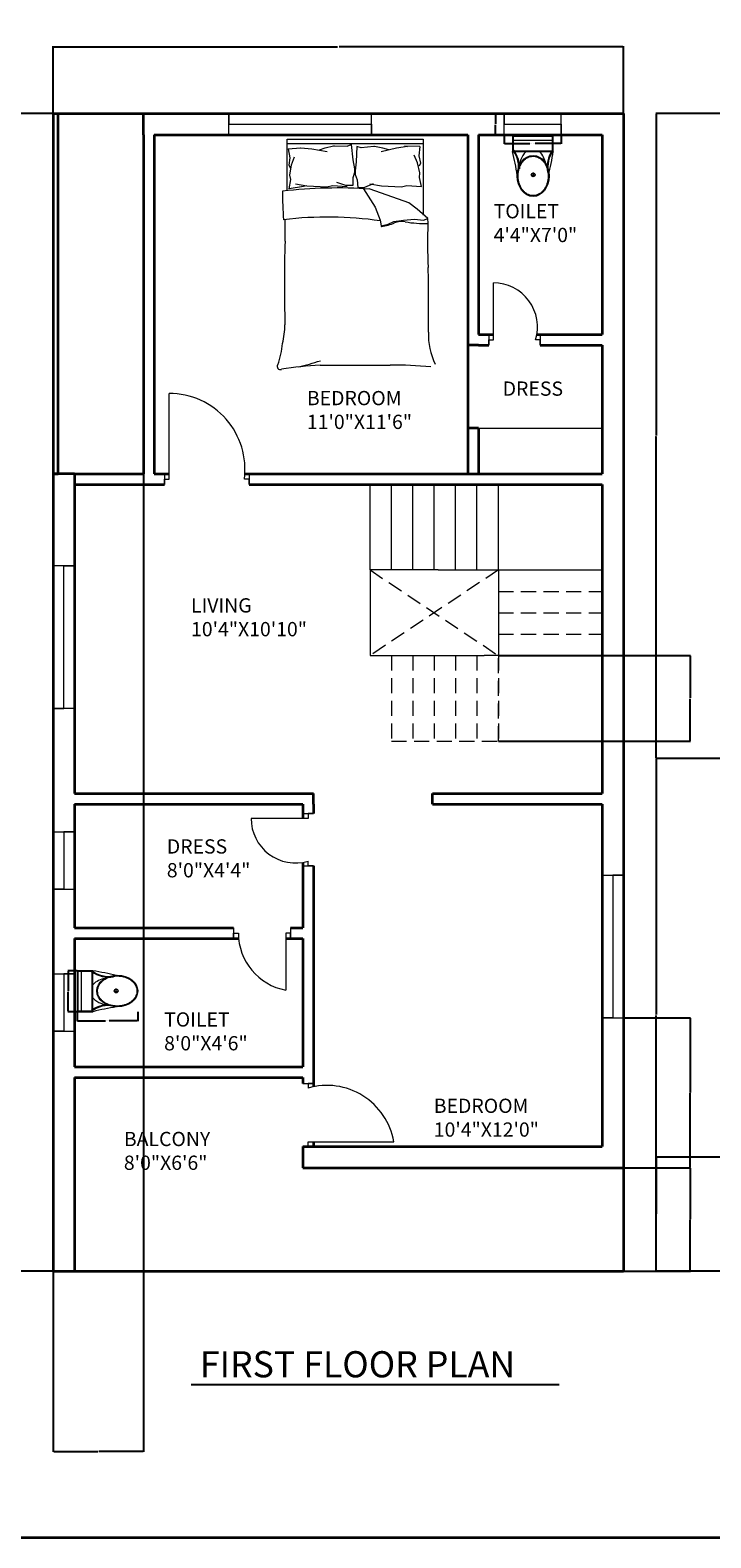
# Model space of a CAD drawing. Units: inches. Extents: x 1911 to 3278, y 2022 to 3108.
# Tile 9 of 13: x 2298 to 2585, y 2022 to 2656. Entities that reach past the tile are written whole.
import ezdxf

# ---------------------------------------------------------------- set-up
doc = ezdxf.new("R2010")
doc.units = ezdxf.units.IN
doc.linetypes.add('DASHED2', pattern=[9.525, 6.35, -3.175])
for name, color, linetype, lineweight in [('A-ANNO-DIMS', 2, 'Continuous', 18), ('A-ANNO-TITL', 7, 'Continuous', 25), ('A-ANNO-TTLB', 7, 'Continuous', 35), ('A-AREA-IDEN', 7, 'Continuous', 18), ('A-DOOR', 4, 'Continuous', 18), ('A-FLOR-CASE', 9, 'Continuous', 18), ('A-FLOR-FIXT', 9, 'Continuous', 18), ('A-FLOR-STRS', 7, 'Continuous', 18), ('A-FLOR-STRS-OVHD', 253, 'DASHED2', 13), ('A-FURN', 8, 'Continuous', 13), ('A-GLAZ', 4, 'Continuous', 18), ('A-WALL', 7, 'Continuous', 35)]:
    doc.layers.add(name, color=color, linetype=linetype, lineweight=lineweight)
doc.styles.get("Standard").update_dxf_attribs({"font": 'arial.ttf'})
doc.dimstyles.get("Standard").update_dxf_attribs({"dimtxt": 0.18, "dimasz": 0.18, "dimexe": 0.18, "dimexo": 0.0625, "dimgap": 0.09, "dimtad": 0, "dimtih": 1, "dimtoh": 1, "dimdec": 4, "dimzin": 0, "dimdsep": 46, "dimtxsty": 'Standard', "dimcen": 0.09, "dimadec": 0, "dimazin": 0, "dimtfac": 1, "dimtdec": 4, "dimtofl": 0, "dimtmove": 0, "dimatfit": 3, "dimfxl": 1, "dimtolj": 1, "dimtzin": 0, "dimarcsym": 0})

# ---------------------------------------------------------------- blocks, each defined once
blk = doc.blocks.new('A$C31115884')
for p, q in [((283, 498), (223, 498)), ((258, 466), (258, 523)), ((0, 200), (0, 0)), ((520, 200), (0, 200)), ((520, 0), (520, 200)), ((510, 54), (0, 54)), ((10, 190), (10, 10)), ((510, 190), (10, 190)), ((10, 10), (510, 10)), ((510, 10), (510, 190)), ((0, 0), (520, 0))]:
    blk.add_line(p, q)
blk.add_circle((256, 496), 23.6)
for centre, radius, start, end in [((2778, -205), 2807, 165.4549, 171.7133), ((-295, 403), 365, 324.2091, 9.3499), ((-295, 403), 375, 324.2091, 9.3499), ((139, 406), 293, 315.8436, 2.6563), ((806, 403), 375, 179.2036, 215.7909), ((806, 403), 365, 170.6501, 215.7909), ((3237, 905), 2807, 188.2867, 194.5451), ((384, 406), 293, 190.2774, 224.1564)]:
    blk.add_arc(centre, radius, start, end)
blk.add_ellipse((256, 510), major_axis=(0, -261), ratio=0.772727)
blk.add_open_spline([(256, 259), (263, 259), (270, 260), (288, 262), (299, 265), (320, 273), (330, 278), (350, 291), (360, 299), (378, 316), (386, 326), (402, 347), (409, 358), (421, 383), (427, 395), (436, 422), (440, 436), (445, 465), (447, 480), (448, 509), (448, 524), (445, 553), (443, 568), (436, 596), (432, 610), (422, 636), (416, 649), (402, 672), (395, 683), (379, 703), (370, 712), (351, 728), (341, 735), (321, 746), (310, 751), (289, 757), (278, 759), (256, 761), (245, 761), (223, 757), (212, 754), (191, 746), (181, 741), (161, 728), (151, 720), (133, 703), (125, 693), (110, 672), (103, 660), (90, 636), (85, 623), (76, 596), (72, 582), (67, 553), (66, 538), (64, 509), (65, 494), (68, 465), (70, 450), (77, 422), (81, 408), (91, 382), (97, 370), (111, 346), (118, 335), (135, 316), (144, 307), (162, 291), (172, 284), (193, 273), (203, 269), (225, 262), (236, 260), (250, 259), (253, 259), (256, 259)], degree=3, knots=[0, 0, 0, 0, 0.110105, 0.110105, 0.285049, 0.285049, 0.459994, 0.459994, 0.634938, 0.634938, 0.809882, 0.809882, 0.984827, 0.984827, 1.159771, 1.159771, 1.334715, 1.334715, 1.50966, 1.50966, 1.684604, 1.684604, 1.859549, 1.859549, 2.034493, 2.034493, 2.209437, 2.209437, 2.384382, 2.384382, 2.559326, 2.559326, 2.73427, 2.73427, 2.909215, 2.909215, 3.084159, 3.084159, 3.259103, 3.259103, 3.434048, 3.434048, 3.608992, 3.608992, 3.783936, 3.783936, 3.958881, 3.958881, 4.133825, 4.133825, 4.30877, 4.30877, 4.483714, 4.483714, 4.658658, 4.658658, 4.833603, 4.833603, 5.008547, 5.008547, 5.183491, 5.183491, 5.358436, 5.358436, 5.53338, 5.53338, 5.708324, 5.708324, 5.883269, 5.883269, 6.058213, 6.058213, 6.233158, 6.233158, 6.283185, 6.283185, 6.283185, 6.283185])
blk = doc.blocks.new('WIN-60')
for p, q in [((0, 60), (9, 60)), ((9, 60), (4.5, 60)), ((4.5, 60), (4.5, 0)), ((4.5, 0), (0, 0)), ((0, 0), (9, 0))]:
    blk.add_line(p, q)
blk = doc.blocks.new('WIN-24')
for p, q in [((0, 24), (9, 24)), ((9, 24), (4.5, 24)), ((4.5, 24), (4.5, 0)), ((4.5, 0), (0, 0)), ((0, 0), (9, 0))]:
    blk.add_line(p, q)
blk = doc.blocks.new('DOOR-BED-FF')
for p, q in [((2, 2.25), (2, 38.25)), ((0, 4.5), (0, 0)), ((0, 0), (0, 2.25)), ((0, 2.25), (2, 2.25)), ((35.66, 2.25), (33.66, 2.25)), ((35.66, 4.5), (35.66, 0)), ((35.66, 0), (35.66, 2.25))]:
    blk.add_line(p, q)
blk.add_arc((2, 6.33), 31.92, 352.65052, 90)
blk = doc.blocks.new('DOOR-BATH-FF')
for p, q in [((2, 2.25), (2, 26.25)), ((0, 4.5), (0, 0)), ((0, 0), (0, 2.25)), ((0, 2.25), (2, 2.25)), ((21.7, 2.25), (19.7, 2.25)), ((21.7, 4.5), (21.7, 0)), ((21.7, 0), (21.7, 2.25))]:
    blk.add_line(p, q)
blk.add_arc((2, 7.72), 18.53, 342.82983, 90)
blk = doc.blocks.new('DOOR-BALCONY')
for p, q in [((0, 26.53), (4.5, 26.53)), ((4.5, 26.53), (2.25, 26.53)), ((2.25, 26.53), (2.25, 24.53)), ((2.32, 0), (2.32, 2)), ((2.32, 2), (38.32, 2))]:
    blk.add_line(p, q)
blk.add_arc((10.23, -2.83), 28.5, 9.76334, 106.26632)
blk = doc.blocks.new('DOOR-DRESS-FF')
for p, q in [((24, 20), (0, 20)), ((21.75, 22), (26.25, 22)), ((26.25, 22), (24, 22)), ((24, 22), (24, 20)), ((21.75, 0), (26.25, 0)), ((24, 0), (24, 2)), ((26.25, 0), (24, 0))]:
    blk.add_line(p, q)
blk.add_arc((18.75, 20), 18.75, 180, 286.25091)
blk = doc.blocks.new('DOOR-ENSUITE-FF')
for p, q in [((0, 26.25), (0, 21.75)), ((23.93, 26.25), (23.93, 21.75)), ((0, 21.75), (0, 24)), ((0, 24), (0, 24)), ((0, 24), (2, 24)), ((23.93, 24), (21.93, 24)), ((21.93, 24), (21.93, 0)), ((23.93, 21.75), (23.93, 24))]:
    blk.add_line(p, q)
blk.add_arc((26.42, 24), 24.42, 180, 259.41225)
blk = doc.blocks.new('BED-DOUBLE')
for p, q in [((4.17, 75.16), (4.17, 96.87)), ((4.17, 96.87), (61.46, 96.87)), ((61.46, 96.87), (61.46, 64.97)), ((4.17, 95.03), (61.46, 95.03)), ((4.67, 92.87), (9.81, 93.27)), ((4.67, 92.9), (5.36, 89.08)), ((5.36, 89.08), (4.84, 85.96)), ((6.06, 86.14), (7.27, 89.43)), ((9.81, 93.27), (9.93, 93.24)), ((9.93, 93.24), (14.52, 92.9)), ((14.52, 92.9), (21.1, 91.68)), ((17.81, 92.38), (20.24, 93.24)), ((20.24, 93.24), (23.7, 94.11)), ((23.7, 94.11), (24.09, 94.11)), ((24.09, 94.11), (29.42, 93.94)), ((29.42, 93.94), (31.15, 94.63)), ((31.15, 94.63), (31.84, 88.22)), ((33.54, 93.88), (33.25, 87.44)), ((35.31, 93.3), (33.54, 93.88)), ((40.62, 93.81), (35.31, 93.3)), ((41.01, 93.83), (40.62, 93.81)), ((44.52, 93.18), (41.01, 93.83)), ((50.25, 93.19), (43.75, 91.57)), ((47, 92.47), (44.52, 93.18)), ((54.8, 93.82), (50.25, 93.19)), ((60.08, 93.81), (53.6, 93.92)), ((53.6, 93.92), (54.8, 93.82)), ((59.12, 86.97), (57.7, 90.18)), ((60.08, 93.81), (59.62, 89.96)), ((59.62, 89.96), (60.34, 86.88)), ((4.84, 85.96), (5.54, 84.75)), ((5.36, 81.8), (6.06, 86.14)), ((31.84, 88.22), (32.54, 84.4)), ((32.54, 82.84), (31.84, 80.59)), ((32.54, 84.4), (32.54, 82.84)), ((33.25, 87.44), (32.79, 83.59)), ((32.79, 83.59), (32.89, 82.03)), ((60.08, 82.69), (59.12, 86.97)), ((60.34, 86.88), (59.72, 85.62)), ((59.85, 80.77), (60.08, 82.69)), ((5.02, 76.08), (5.71, 79.9)), ((11.13, 76.95), (5.02, 76.08)), ((5.71, 79.9), (5.36, 81.8)), ((7.65, 78.14), (12.48, 77.34)), ((12.48, 77.34), (11.13, 76.95)), ((12.48, 77.34), (20.89, 76.82)), ((20.89, 76.82), (23.24, 77.49)), ((23.24, 77.49), (29.39, 77)), ((28.9, 77.37), (25.13, 78.68)), ((31.84, 77.37), (28.9, 77.37)), ((31.84, 80.59), (31.84, 77.37)), ((32.89, 82.03), (33.72, 79.83)), ((33.72, 79.83), (33.93, 76.62)), ((33.93, 76.62), (36.87, 76.8)), ((36.87, 76.8), (40.55, 78.34)), ((39.04, 78.14), (43.87, 77.34)), ((43.87, 77.34), (52.28, 76.82)), ((52.28, 76.82), (54.63, 77.49)), ((54.63, 77.49), (60.78, 77)), ((60.78, 77), (59.85, 80.77)), ((36.28, 76.03), (41.3, 68.25)), ((48.73, 72.52), (38.73, 76.03)), ((55.41, 70.1), (48.73, 72.52)), ((58.94, 67.51), (55.41, 70.1)), ((41.3, 68.25), (43.34, 62.87)), ((63.38, 63.61), (58.94, 67.51)), ((61.54, 62.87), (63.38, 63.61)), ((63.48, 61.52), (63.38, 63.61, 4.64)), ((43.34, 62.87), (43.71, 60.45)), ((43.71, 60.45), (46.68, 61.2)), ((46.68, 61.2), (49.1, 62.31)), ((49.1, 62.31), (53.18, 62.87)), ((53.18, 62.87), (57.82, 63.24)), ((57.82, 63.24), (61.54, 62.87)), ((18.06, 1.87), (47.57, 1.87))]:
    blk.add_line(p, q)
for centre, radius, start, end in [((25.61, -121.38), 197.77, 86.08655, 96.78213), ((102.1, 72.78), 99.87, 178.72178, 185.60397), ((21.29, -90.53), 154.68, 81.78449, 96.90062), ((-200.58, 59.5), 203.94, 358.4762, 1.00819), ((43.92, 60.38), 0.221, 160.24637, 271.13765), ((37.35, 95.1), 35.55, 280.66171, 289.88058), ((52.44, 54.83), 7.46, 78.6608, 113.73842), ((61.53, 104.85), 43.38, 259.87628, 272.56571), ((218.51, 53.34), 155.25, 176.97912, 183.83645), ((581.23, 36.19), 578.22, 178.22771, 181.71854), ((-5405.34, 15.56), 5469.02, 0.00217, 0.28689), ((-32.25, 19.53), 35.53, 346.06484, 358.91125), ((91.3, 14.55), 27.65, 177.47136, 206.46809), ((-25.97, 12.62), 28.25, 337.97508, 356.652), ((1.3, 1.3), 1.31, 146.17358, 293.47814), ((25.69, -143.9), 145.97, 92.99578, 99.40907), ((-20.65, 125.3), 127.63, 283.38322, 287.70533), ((49.34, -157.62), 159.5, 84.4998, 90.63509)]:
    blk.add_arc(centre, radius, start, end)
blk = doc.blocks.new('STAIR-PLAN-FF')
for p, q in [((0, 36), (0, 72)), ((9, 36), (9, 72)), ((18, 36), (18, 72)), ((27, 36), (27, 72)), ((36, 36), (36, 72)), ((45, 36), (45, 72)), ((54, 36), (54, 72)), ((28.63, 36), (0, 36)), ((0, 36), (0, 0)), ((28.63, 36), (97.65, 36)), ((54, 36), (54, 0)), ((54, 36), (54, 27)), ((0, 0), (48, 0)), ((54, 0), (48, 0))]:
    blk.add_line(p, q)
blk = doc.blocks.new('STAIR-BEYOND-FF')
for p, q in [((54, 72), (0, 36)), ((0, 72), (54, 36)), ((54, 72), (54, 63)), ((54, 63), (97.65, 63)), ((54, 54), (97.65, 54)), ((54, 45), (97.65, 45)), ((9, 36), (9, 0)), ((18, 36), (18, 0)), ((27, 36), (27, 0)), ((36, 36), (36, 0)), ((45, 36), (45, 0)), ((54, 36), (97.65, 36)), ((54, 0), (54, 36)), ((54, 36), (54, 0)), ((9, 0), (54, 0))]:
    blk.add_line(p, q)
blk = doc.blocks.new('*D26')
at = {"layer": 'A-ANNO-DIMS', "color": 0, "lineweight": -2, "transparency": 16777216}
for p, q in [((2497.89, 2611.81), (2497.89, 2608.09)), ((2498.07, 2608.27), (2508.77, 2608.27)), ((2521.71, 2608.27), (2511.01, 2608.27)), ((2521.89, 2611.81), (2521.89, 2608.09))]:
    blk.add_line(p, q, dxfattribs=at)
at = {"layer": 'A-ANNO-DIMS', "color": 0, "transparency": 16777216}
for points in [[(2498.07, 2608.3), (2498.07, 2608.24), (2497.89, 2608.27)], [(2521.71, 2608.3), (2521.71, 2608.24), (2521.89, 2608.27)]]:
    blk.add_solid(points, dxfattribs=at)
at = {"layer": 'Defpoints', "color": 0, "transparency": 16777216}
for p in [(2497.89, 2611.87), (2497.89, 2608.27), (2521.89, 2611.87)]:
    blk.add_point(p, dxfattribs=at)
at = {"layer": 'A-ANNO-DIMS', "color": 0, "transparency": 16777216, "insert": (2509.89, 2608.27), "char_height": 0.18, "attachment_point": 5}
blk.add_mtext('\\A1;WINDOW 24 TYP.', dxfattribs=at)
blk = doc.blocks.new('*D27')
at = {"layer": 'A-ANNO-DIMS', "color": 0, "lineweight": -2, "transparency": 16777216}
for p, q in [((2497.83, 2620.87), (2494.11, 2620.87)), ((2494.29, 2620.69), (2494.29, 2616.56)), ((2494.29, 2612.05), (2494.29, 2616.19)), ((2497.83, 2611.87), (2494.11, 2611.87))]:
    blk.add_line(p, q, dxfattribs=at)
at = {"layer": 'A-ANNO-DIMS', "color": 0, "transparency": 16777216}
for points in [[(2494.26, 2620.69), (2494.32, 2620.69), (2494.29, 2620.87)], [(2494.26, 2612.05), (2494.32, 2612.05), (2494.29, 2611.87)]]:
    blk.add_solid(points, dxfattribs=at)
at = {"layer": 'Defpoints', "color": 0, "transparency": 16777216}
for p in [(2494.29, 2620.87), (2497.89, 2620.87), (2497.89, 2611.87)]:
    blk.add_point(p, dxfattribs=at)
at = {"layer": 'A-ANNO-DIMS', "color": 0, "transparency": 16777216, "insert": (2494.29, 2616.37), "char_height": 0.18, "attachment_point": 5}
blk.add_mtext('\\A1;9 TYP.', dxfattribs=at)
blk = doc.blocks.new('*D34')
at = {"layer": 'A-ANNO-DIMS', "color": 0, "lineweight": -2, "transparency": 16777216}
for p, q in [((2318.18, 2242.98), (2318.18, 2239.04)), ((2318.36, 2239.22), (2330.15, 2239.22)), ((2343.48, 2239.22), (2331.7, 2239.22)), ((2343.66, 2242.98), (2343.66, 2239.04))]:
    blk.add_line(p, q, dxfattribs=at)
at = {"layer": 'A-ANNO-DIMS', "color": 0, "transparency": 16777216}
for points in [[(2318.36, 2239.25), (2318.36, 2239.19), (2318.18, 2239.22)], [(2343.48, 2239.25), (2343.48, 2239.19), (2343.66, 2239.22)]]:
    blk.add_solid(points, dxfattribs=at)
at = {"layer": 'Defpoints', "color": 0, "transparency": 16777216}
for p in [(2318.18, 2243.04), (2343.66, 2243.04), (2343.66, 2239.22)]:
    blk.add_point(p, dxfattribs=at)
at = {"layer": 'A-ANNO-DIMS', "color": 0, "transparency": 16777216, "insert": (2330.92, 2239.22), "char_height": 0.18, "attachment_point": 5}
blk.add_mtext('\\A1;WC 25 TYP.', dxfattribs=at)
blk = doc.blocks.new('*D35')
at = {"layer": 'A-ANNO-DIMS', "color": 0, "lineweight": -2, "transparency": 16777216}
for p, q in [((2318.12, 2260.24), (2314.18, 2260.24)), ((2314.36, 2260.06), (2314.36, 2251.82)), ((2314.36, 2243.22), (2314.36, 2251.46)), ((2318.12, 2243.04), (2314.18, 2243.04))]:
    blk.add_line(p, q, dxfattribs=at)
at = {"layer": 'A-ANNO-DIMS', "color": 0, "transparency": 16777216}
for points in [[(2314.33, 2260.06), (2314.39, 2260.06), (2314.36, 2260.24)], [(2314.33, 2243.22), (2314.39, 2243.22), (2314.36, 2243.04)]]:
    blk.add_solid(points, dxfattribs=at)
at = {"layer": 'Defpoints', "color": 0, "transparency": 16777216}
for p in [(2318.18, 2260.24), (2314.36, 2243.04), (2318.18, 2243.04)]:
    blk.add_point(p, dxfattribs=at)
at = {"layer": 'A-ANNO-DIMS', "color": 0, "transparency": 16777216, "insert": (2314.36, 2251.64), "char_height": 0.18, "attachment_point": 5}
blk.add_mtext('\\A1;17 TYP.', dxfattribs=at)
blk = doc.blocks.new('*D75')
at = {"layer": 'A-ANNO-DIMS', "color": 0, "lineweight": -2, "transparency": 16777216}
for p, q in [((2308.12, 2620.94), (2308.12, 2649.15)), ((2308.3, 2648.97), (2427.83, 2648.97)), ((2547.94, 2648.97), (2428.41, 2648.97)), ((2548.12, 2620.94), (2548.12, 2649.15))]:
    blk.add_line(p, q, dxfattribs=at)
at = {"layer": 'A-ANNO-DIMS', "color": 0, "transparency": 16777216}
for points in [[(2308.3, 2649), (2308.3, 2648.94), (2308.12, 2648.97)], [(2547.94, 2649), (2547.94, 2648.94), (2548.12, 2648.97)]]:
    blk.add_solid(points, dxfattribs=at)
at = {"layer": 'Defpoints', "color": 0, "transparency": 16777216}
for p in [(2548.12, 2648.97), (2308.12, 2620.87), (2548.12, 2620.87)]:
    blk.add_point(p, dxfattribs=at)
at = {"layer": 'A-ANNO-DIMS', "color": 0, "transparency": 16777216, "insert": (2428.12, 2648.97), "char_height": 0.18, "attachment_point": 5}
blk.add_mtext('\\A1;240', dxfattribs=at)
blk = doc.blocks.new('*D76')
at = {"layer": 'A-ANNO-DIMS', "color": 0, "lineweight": -2, "transparency": 16777216}
for p, q in [((2308.06, 2620.87), (2279.84, 2620.87)), ((2280.02, 2620.69), (2280.02, 2377.56)), ((2280.02, 2134.05), (2280.02, 2377.19)), ((2308.06, 2133.87), (2279.84, 2133.87))]:
    blk.add_line(p, q, dxfattribs=at)
at = {"layer": 'A-ANNO-DIMS', "color": 0, "transparency": 16777216}
for points in [[(2279.99, 2620.69), (2280.05, 2620.69), (2280.02, 2620.87)], [(2279.99, 2134.05), (2280.05, 2134.05), (2280.02, 2133.87)]]:
    blk.add_solid(points, dxfattribs=at)
at = {"layer": 'Defpoints', "color": 0, "transparency": 16777216}
for p in [(2280.02, 2620.87), (2308.12, 2620.87), (2308.12, 2133.87)]:
    blk.add_point(p, dxfattribs=at)
at = {"layer": 'A-ANNO-DIMS', "color": 0, "transparency": 16777216, "insert": (2280.02, 2377.37), "char_height": 0.18, "attachment_point": 5}
blk.add_mtext('\\A1;487', dxfattribs=at)
blk = doc.blocks.new('*D77')
at = {"layer": 'A-ANNO-DIMS', "color": 0, "lineweight": -2, "transparency": 16777216}
for p, q in [((2308.12, 2620.81), (2308.12, 2057.89)), ((2346.12, 2620.81), (2346.12, 2057.89)), ((2308.3, 2058.07), (2326.9, 2058.07)), ((2345.94, 2058.07), (2327.34, 2058.07))]:
    blk.add_line(p, q, dxfattribs=at)
at = {"layer": 'A-ANNO-DIMS', "color": 0, "transparency": 16777216}
for points in [[(2308.3, 2058.1), (2308.3, 2058.04), (2308.12, 2058.07)], [(2345.94, 2058.1), (2345.94, 2058.04), (2346.12, 2058.07)]]:
    blk.add_solid(points, dxfattribs=at)
at = {"layer": 'Defpoints', "color": 0, "transparency": 16777216}
for p in [(2308.12, 2620.87), (2346.12, 2620.87), (2346.12, 2058.07)]:
    blk.add_point(p, dxfattribs=at)
at = {"layer": 'A-ANNO-DIMS', "color": 0, "transparency": 16777216, "insert": (2327.12, 2058.07), "char_height": 0.18, "attachment_point": 5}
blk.add_mtext('\\A1;38', dxfattribs=at)
blk = doc.blocks.new('*D78')
at = {"layer": 'A-ANNO-DIMS', "color": 0, "lineweight": -2, "transparency": 16777216}
for p, q in [((2548.18, 2177.37), (2576.4, 2177.37)), ((2576.22, 2177.19), (2576.22, 2155.81)), ((2576.22, 2134.05), (2576.22, 2155.44)), ((2548.18, 2133.87), (2576.4, 2133.87))]:
    blk.add_line(p, q, dxfattribs=at)
at = {"layer": 'A-ANNO-DIMS', "color": 0, "transparency": 16777216}
for points in [[(2576.19, 2177.19), (2576.25, 2177.19), (2576.22, 2177.37)], [(2576.19, 2134.05), (2576.25, 2134.05), (2576.22, 2133.87)]]:
    blk.add_solid(points, dxfattribs=at)
at = {"layer": 'Defpoints', "color": 0, "transparency": 16777216}
for p in [(2548.12, 2177.37), (2576.22, 2177.37), (2548.12, 2133.87)]:
    blk.add_point(p, dxfattribs=at)
at = {"layer": 'A-ANNO-DIMS', "color": 0, "transparency": 16777216, "insert": (2576.22, 2155.62), "char_height": 0.18, "attachment_point": 5}
blk.add_mtext('\\A1;43.5', dxfattribs=at)
blk = doc.blocks.new('*D79')
at = {"layer": 'A-ANNO-DIMS', "color": 0, "lineweight": -2, "transparency": 16777216}
for p, q in [((2548.18, 2240.47), (2576.4, 2240.47)), ((2576.22, 2240.29), (2576.22, 2209.1)), ((2576.22, 2177.55), (2576.22, 2208.74)), ((2548.18, 2177.37), (2576.4, 2177.37))]:
    blk.add_line(p, q, dxfattribs=at)
at = {"layer": 'A-ANNO-DIMS', "color": 0, "transparency": 16777216}
for points in [[(2576.19, 2240.29), (2576.25, 2240.29), (2576.22, 2240.47)], [(2576.19, 2177.55), (2576.25, 2177.55), (2576.22, 2177.37)]]:
    blk.add_solid(points, dxfattribs=at)
at = {"layer": 'Defpoints', "color": 0, "transparency": 16777216}
for p in [(2548.12, 2240.47), (2576.22, 2240.47), (2548.12, 2177.37)]:
    blk.add_point(p, dxfattribs=at)
at = {"layer": 'A-ANNO-DIMS', "color": 0, "transparency": 16777216, "insert": (2576.22, 2208.92), "char_height": 0.18, "attachment_point": 5}
blk.add_mtext('\\A1;63.09', dxfattribs=at)
blk = doc.blocks.new('*D80')
at = {"layer": 'A-ANNO-DIMS', "color": 0, "lineweight": -2, "transparency": 16777216}
for p, q in [((2495.53, 2392.87), (2576.4, 2392.87)), ((2576.22, 2392.69), (2576.22, 2375.06)), ((2576.22, 2357.05), (2576.22, 2374.69)), ((2495.53, 2356.87), (2576.4, 2356.87))]:
    blk.add_line(p, q, dxfattribs=at)
at = {"layer": 'A-ANNO-DIMS', "color": 0, "transparency": 16777216}
for points in [[(2576.19, 2392.69), (2576.25, 2392.69), (2576.22, 2392.87)], [(2576.19, 2357.05), (2576.25, 2357.05), (2576.22, 2356.87)]]:
    blk.add_solid(points, dxfattribs=at)
at = {"layer": 'Defpoints', "color": 0, "transparency": 16777216}
for p in [(2495.47, 2392.87), (2495.47, 2356.87), (2576.22, 2356.87)]:
    blk.add_point(p, dxfattribs=at)
at = {"layer": 'A-ANNO-DIMS', "color": 0, "transparency": 16777216, "insert": (2576.22, 2374.87), "char_height": 0.18, "attachment_point": 5}
blk.add_mtext('\\A1;36', dxfattribs=at)
blk = doc.blocks.new('*D83')
at = {"layer": 'A-ANNO-DIMS', "color": 0, "lineweight": -2, "transparency": 16777216}
for p, q in [((2633.29, 2620.87), (2561.76, 2620.87)), ((2561.94, 2620.69), (2561.94, 2485.38)), ((2561.94, 2349.71), (2561.94, 2485.02)), ((2593.28, 2349.53), (2561.76, 2349.53))]:
    blk.add_line(p, q, dxfattribs=at)
at = {"layer": 'A-ANNO-DIMS', "color": 0, "transparency": 16777216}
for points in [[(2561.91, 2620.69), (2561.97, 2620.69), (2561.94, 2620.87)], [(2561.91, 2349.71), (2561.97, 2349.71), (2561.94, 2349.53)]]:
    blk.add_solid(points, dxfattribs=at)
at = {"layer": 'Defpoints', "color": 0, "transparency": 16777216}
for p in [(2561.94, 2620.87), (2633.35, 2620.87), (2593.34, 2349.53)]:
    blk.add_point(p, dxfattribs=at)
at = {"layer": 'A-ANNO-DIMS', "color": 0, "transparency": 16777216, "insert": (2561.94, 2485.2), "char_height": 0.18, "attachment_point": 5}
blk.add_mtext('\\A1;271.35', dxfattribs=at)
blk = doc.blocks.new('*D87')
at = {"layer": 'A-ANNO-DIMS', "color": 0, "lineweight": -2, "transparency": 16777216}
for p, q in [((2593.28, 2349.53), (2561.76, 2349.53)), ((2561.94, 2349.35), (2561.94, 2241.88)), ((2561.94, 2134.05), (2561.94, 2241.52)), ((2633.29, 2133.87), (2561.76, 2133.87))]:
    blk.add_line(p, q, dxfattribs=at)
at = {"layer": 'A-ANNO-DIMS', "color": 0, "transparency": 16777216}
for points in [[(2561.91, 2349.35), (2561.97, 2349.35), (2561.94, 2349.53)], [(2561.91, 2134.05), (2561.97, 2134.05), (2561.94, 2133.87)]]:
    blk.add_solid(points, dxfattribs=at)
at = {"layer": 'Defpoints', "color": 0, "transparency": 16777216}
for p in [(2593.34, 2349.53), (2561.94, 2133.87), (2633.35, 2133.87)]:
    blk.add_point(p, dxfattribs=at)
at = {"layer": 'A-ANNO-DIMS', "color": 0, "transparency": 16777216, "insert": (2561.94, 2241.7), "char_height": 0.18, "attachment_point": 5}
blk.add_mtext('\\A1;215.65', dxfattribs=at)
blk = doc.blocks.new('*D88')
at = {"layer": 'A-ANNO-DIMS', "color": 0, "lineweight": -2, "transparency": 16777216}
for p, q in [((2879.79, 2181.87), (2561.76, 2181.87)), ((2561.94, 2181.69), (2561.94, 2158.06)), ((2561.94, 2134.05), (2561.94, 2157.69)), ((2879.79, 2133.87), (2561.76, 2133.87))]:
    blk.add_line(p, q, dxfattribs=at)
at = {"layer": 'A-ANNO-DIMS', "color": 0, "transparency": 16777216}
for points in [[(2561.91, 2181.69), (2561.97, 2181.69), (2561.94, 2181.87)], [(2561.91, 2134.05), (2561.97, 2134.05), (2561.94, 2133.87)]]:
    blk.add_solid(points, dxfattribs=at)
at = {"layer": 'Defpoints', "color": 0, "transparency": 16777216}
for p in [(2561.94, 2181.87), (2879.85, 2181.87), (2879.85, 2133.87)]:
    blk.add_point(p, dxfattribs=at)
at = {"layer": 'A-ANNO-DIMS', "color": 0, "transparency": 16777216, "insert": (2561.94, 2157.87), "char_height": 0.18, "attachment_point": 5}
blk.add_mtext('\\A1;48', dxfattribs=at)

msp = doc.modelspace()

# ---------------------------------------------------------------- linework, layer by layer
at = {"layer": 'A-ANNO-TITL'}
msp.add_line((2366.1029, 2086.1736), (2521.0254, 2086.1736), dxfattribs=at)
at = {"layer": 'A-ANNO-TTLB'}
msp.add_lwpolyline([(1911.3875, 3108.0628), (3278.3142, 3108.0628), (3278.3142, 2021.7237), (1911.3875, 2021.7237)], close=True, dxfattribs=at)
at = {"layer": 'A-FLOR-CASE'}
msp.add_line((2482.6192, 2488.532), (2539.1192, 2488.532), dxfattribs=at)
at = {"layer": 'A-WALL'}
for p, q in [((2308.1192, 2620.8733), (2548.1192, 2620.8733)), ((2308.1192, 2620.8733), (2308.1192, 2133.8733)), ((2310.1192, 2473.8733), (2310.1192, 2620.8733)), ((2346.1192, 2611.8733), (2346.1192, 2620.8733)), ((2548.1192, 2620.8733), (2548.1192, 2133.8733)), ((2346.1192, 2611.8733), (2346.1192, 2469.3733)), ((2350.6192, 2611.8733), (2350.6192, 2469.3733)), ((2350.6192, 2611.8733), (2482.6192, 2611.8733)), ((2482.6192, 2611.8733), (2482.6192, 2469.3733)), ((2487.1192, 2611.8733), (2487.1192, 2527.8733)), ((2487.1192, 2611.8733), (2539.1192, 2611.8733)), ((2539.1192, 2611.8733), (2539.1192, 2527.8733)), ((2487.1192, 2527.8733), (2493.4153, 2527.8733)), ((2511.6631, 2527.8733), (2539.1192, 2527.8733)), ((2487.1192, 2523.3733), (2482.6192, 2523.3733)), ((2487.1192, 2523.3733), (2491.4153, 2523.3733)), ((2513.1192, 2523.3733), (2539.1192, 2523.3733)), ((2539.1192, 2523.3733), (2539.1192, 2469.3733)), ((2487.1192, 2488.532), (2482.6192, 2488.532)), ((2487.1192, 2488.532), (2487.1192, 2469.3733)), ((2310.1192, 2469.3733), (2310.1192, 2473.8733)), ((2317.1192, 2469.3733), (2308.1192, 2469.3733)), ((2308.1192, 2469.3733), (2310.1192, 2469.3733)), ((2317.1192, 2469.3733), (2317.1192, 2334.8733)), ((2317.1192, 2469.3733), (2346.1192, 2469.3733)), ((2350.6192, 2469.3733), (2356.9015, 2469.3733)), ((2388.7659, 2469.3733), (2539.1192, 2469.3733)), ((2317.1192, 2464.8733), (2354.9015, 2464.8733)), ((2390.5564, 2464.8733), (2539.1192, 2464.8733)), ((2539.1192, 2464.8733), (2539.1192, 2334.8733)), ((2317.1192, 2334.8733), (2417.6192, 2334.8733)), ((2417.6192, 2330.3733), (2417.6192, 2334.8733)), ((2467.7746, 2330.3733), (2467.7746, 2334.8733)), ((2467.7746, 2334.8733), (2539.1192, 2334.8733)), ((2317.1192, 2330.3733), (2413.1192, 2330.3733)), ((2317.1192, 2330.3733), (2317.1192, 2278.3733)), ((2413.1192, 2330.3733), (2413.1192, 2324.3763)), ((2417.6192, 2330.3733), (2417.6192, 2326.3763)), ((2467.7746, 2330.3733), (2539.1192, 2330.3733)), ((2539.1192, 2330.3733), (2539.1192, 2186.3733)), ((2413.1192, 2305.8652), (2413.1192, 2278.3733)), ((2417.6192, 2304.3733), (2417.6192, 2215.3733)), ((2317.1192, 2278.3733), (2384.0391, 2278.3733)), ((2407.9686, 2278.3733), (2413.1192, 2278.3733)), ((2317.1192, 2273.8733), (2386.143, 2273.8733)), ((2317.1192, 2273.8733), (2317.1192, 2219.8733)), ((2405.9686, 2273.8733), (2413.1192, 2273.8733)), ((2413.1192, 2273.8733), (2413.1192, 2219.8733)), ((2317.1192, 2219.8733), (2413.1192, 2219.8733)), ((2317.1192, 2215.3733), (2413.1192, 2215.3733)), ((2317.1192, 2215.3733), (2317.1192, 2133.8733)), ((2413.1192, 2215.3733), (2413.1192, 2212.8991)), ((2417.6192, 2215.3733), (2417.6192, 2211.4574)), ((2417.6192, 2188.3733), (2417.6192, 2186.3733)), ((2413.1192, 2186.3733), (2539.1192, 2186.3733)), ((2413.1192, 2186.3733), (2413.1192, 2177.3733)), ((2413.1192, 2177.3733), (2539.1192, 2177.3733)), ((2539.1192, 2177.3733), (2548.1192, 2177.3733)), ((2308.1192, 2133.8733), (2548.1192, 2133.8733))]:
    msp.add_line(p, q, dxfattribs=at)

# ---------------------------------------------------------------- block references
at = {"layer": 'A-DOOR'}
for name, p in [('DOOR-BATH-FF', (2491.415, 2523.373)), ('DOOR-BED-FF', (2354.901, 2464.873)), ('DOOR-DRESS-FF', (2391.369, 2304.373)), ('DOOR-ENSUITE-FF', (2384.039, 2252.123)), ('DOOR-BALCONY', (2413.119, 2186.373))]:
    msp.add_blockref(name, p, dxfattribs=at)
at = {"layer": 'A-FLOR-FIXT', "xscale": 0.0330640103915726, "yscale": 0.0330640103915726, "zscale": 0.0330640103915726}
for p, rotation in [((2518.5939, 2611.49), 179.9999999999999), ((2318.184, 2260.237), 269.9999999999999)]:
    msp.add_blockref('A$C31115884', p, dxfattribs=dict(at, rotation=rotation))
at = {"layer": 'A-FLOR-STRS'}
msp.add_blockref('STAIR-PLAN-FF', (2441.47, 2392.873), dxfattribs=at)
at = {"layer": 'A-FLOR-STRS-OVHD'}
msp.add_blockref('STAIR-BEYOND-FF', (2441.47, 2356.873), dxfattribs=at)
at = {"layer": 'A-FURN'}
msp.add_blockref('BED-DOUBLE', (2402.38, 2513.1719), dxfattribs=at)
at = {"layer": 'A-GLAZ'}
for name, p, rotation in [('WIN-60', (2442.0665, 2611.8729), 90.00000000000296), ('WIN-24', (2521.8929, 2611.8729), 90.00000000000595), ('WIN-60', (2317.1196, 2430.5886), 180)]:
    msp.add_blockref(name, p, dxfattribs=dict(at, rotation=rotation))
for name, p in [('WIN-24', (2308.1188, 2294.6461)), ('WIN-60', (2539.1188, 2240.4658)), ('WIN-24', (2308.1188, 2234.9197))]:
    msp.add_blockref(name, p, dxfattribs=at)

# ---------------------------------------------------------------- texts
at = {"layer": 'A-ANNO-TITL', "insert": (2369.835, 2100.2435), "char_height": 11, "attachment_point": 1}
msp.add_mtext_dynamic_manual_height_columns('FIRST FLOOR PLAN', width=276.581827, gutter_width=12.5, heights=[0], dxfattribs=at)
at = {"layer": 'A-AREA-IDEN', "char_height": 6, "attachment_point": 1}
for s, width, insert in [('TOILET\\P4\'4"X7\'0"', 78.589542, (2493.4967, 2582.7867)), ('DRESS', 50.81284, (2497.3064, 2508.159)), ('BEDROOM\\P11\'0"X11\'6"', 78.162095, (2414.8816, 2504.1782)), ('LIVING\\P10\'4"X10\'10"', 75.36049, (2366.1094, 2416.9738)), ('DRESS\\P8\'0"X4\'4"', 106.539489, (2355.917, 2315.5699)), ('TOILET\\P8\'0"X4\'6"', 68.774179, (2354.7789, 2242.7856)), ('BEDROOM\\P10\'4"X12\'0"', 103.209117, (2468.2967, 2206.4723)), ('BALCONY\\P8\'0"X6\'6"', 113.601364, (2337.8375, 2192.5161))]:
    msp.add_mtext_dynamic_manual_height_columns(s, width=width, gutter_width=12.5, heights=[0], dxfattribs=dict(at, insert=insert))

# ---------------------------------------------------------------- dimensions: what is measured, and where the dimension line sits
at = {"layer": 'A-ANNO-DIMS'}
for base, p2, picture, middle in [((2548.1192, 2648.9733), (2548.1192, 2620.8733), '*D75', (2428.1192, 2648.9733)), ((2346.1192, 2058.0736), (2346.1192, 2620.8733), '*D77', (2327.1192, 2058.0736))]:
    dim = msp.add_linear_dim(base=base, p1=(2308.1192, 2620.8733), p2=p2, dimstyle='Standard', override={"dimdec": 0, "dimlfac": 1, "dimrnd": 0, "dimzin": 0, "dimdsep": 46, "dimlunit": 2}, dxfattribs=at)
    dim.commit()
    dim.dimension.update_dxf_attribs({"geometry": picture, "text_midpoint": middle})
for base, p1, p2, override, picture, middle in [((2280.0192, 2620.8733), (2308.1192, 2133.8733), (2308.1192, 2620.8733), {"dimdec": 0, "dimlfac": 1, "dimrnd": 0, "dimzin": 0, "dimdsep": 46, "dimlunit": 2}, '*D76', (2280.0192, 2377.3733)), ((2561.9449, 2620.8733), (2593.3449, 2349.5267), (2633.3539, 2620.8733), {"dimdec": 2, "dimlfac": 1, "dimrnd": 0, "dimzin": 0, "dimdsep": 46, "dimlunit": 2}, '*D83', (2561.9449, 2485.2)), ((2576.2192, 2356.8733), (2495.4699, 2392.8733), (2495.4699, 2356.8733), {"dimdec": 0, "dimlfac": 1, "dimrnd": 0, "dimzin": 0, "dimdsep": 46, "dimlunit": 2}, '*D80', (2576.2192, 2374.8733)), ((2561.9449, 2133.8733), (2593.3449, 2349.5267), (2633.3539, 2133.8733), {"dimdec": 2, "dimlfac": 1, "dimrnd": 0, "dimzin": 0, "dimdsep": 46, "dimlunit": 2}, '*D87', (2561.9449, 2241.7)), ((2576.2192, 2240.4661), (2548.1192, 2177.3733), (2548.1192, 2240.4661), {"dimdec": 2, "dimlfac": 1, "dimrnd": 0, "dimzin": 0, "dimdsep": 46, "dimlunit": 2}, '*D79', (2576.2192, 2208.9197)), ((2561.9449, 2181.8733), (2879.8539, 2133.8733), (2879.8539, 2181.8733), {"dimdec": 0, "dimlfac": 1, "dimrnd": 0, "dimzin": 0, "dimdsep": 46, "dimlunit": 2}, '*D88', (2561.9449, 2157.8733)), ((2576.2192, 2177.3733), (2548.1192, 2133.8733), (2548.1192, 2177.3733), {"dimdec": 1, "dimlfac": 1, "dimrnd": 0, "dimzin": 0, "dimdsep": 46, "dimlunit": 2}, '*D78', (2576.2192, 2155.6233))]:
    dim = msp.add_linear_dim(base=base, p1=p1, p2=p2, angle=90, dimstyle='Standard', override=override, dxfattribs=at)
    dim.commit()
    dim.dimension.update_dxf_attribs({"geometry": picture, "text_midpoint": middle})
for base, p1, p2, angle, text, picture, middle in [((2494.2927, 2620.8733), (2497.8927, 2611.8733), (2497.8927, 2620.8733), 90, '<> TYP.', '*D27', (2494.2927, 2616.3733)), ((2497.8927, 2608.2733), (2521.8927, 2611.8733), (2497.8927, 2611.8733), 180, 'WINDOW <> TYP.', '*D26', (2509.8927, 2608.2733)), ((2314.3623, 2243.0437), (2318.184, 2260.237), (2318.184, 2243.0437), 270, '<> TYP.', '*D35', (2314.3623, 2251.6404))]:
    dim = msp.add_linear_dim(base=base, p1=p1, p2=p2, angle=angle, text=text, dimstyle='Standard', override={"dimdec": 0, "dimlfac": 1, "dimrnd": 0, "dimzin": 0, "dimdsep": 46, "dimlunit": 2}, dxfattribs=at)
    dim.commit()
    dim.dimension.update_dxf_attribs({"geometry": picture, "text_midpoint": middle})
dim = msp.add_linear_dim(base=(2343.6621, 2239.222), p1=(2318.184, 2243.0437), p2=(2343.6621, 2243.0437), text='WC <> TYP.', dimstyle='Standard', override={"dimdec": 0, "dimlfac": 1, "dimrnd": 0, "dimzin": 0, "dimdsep": 46, "dimlunit": 2}, dxfattribs=at)
dim.commit()
dim.dimension.update_dxf_attribs({"geometry": '*D34', "text_midpoint": (2330.9231, 2239.222)})

doc.saveas('drawing.dxf')
